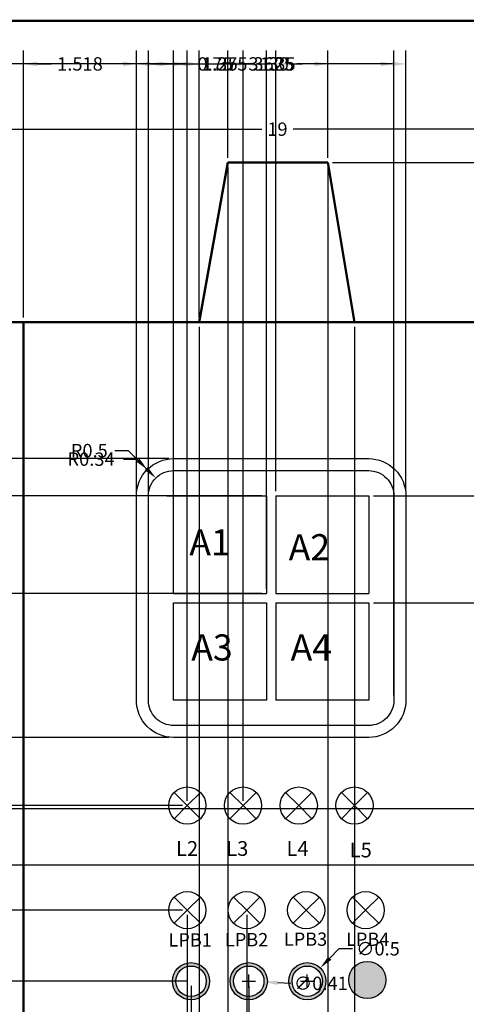
# Model space of a CAD drawing. Units: inches. Extents: x 0 to 33.5, y 0 to 22.4.
# Tile 3 of 6: x 10.7 to 16.8, y 9.2 to 22.4. Entities that reach past the tile are written whole.
import ezdxf
from ezdxf.enums import TextEntityAlignment as Align

# ---------------------------------------------------------------- set-up
doc = ezdxf.new("R2010")
doc.units = ezdxf.units.IN
doc.header["$MEASUREMENT"] = 0
for name, color, linetype, lineweight in [('E-ANNO-DIMS', 2, 'Continuous', 18), ('E-ANNO-TEXT', 7, 'Continuous', 18), ('E-ANNO-TTLB', 7, 'Continuous', 35), ('E-PANL-DEVC', 4, 'Continuous', 25), ('E-PANL-OUTL', 7, 'Continuous', 50), ('E-PANL-PATT', 8, 'Continuous', 13)]:
    doc.layers.add(name, color=color, linetype=linetype, lineweight=lineweight)
doc.layers.add('TITLE', color=7, linetype='Continuous')
doc.styles.add('ITALIC', font='ITALIC')
doc.styles.add('SIMPLEX', font='SIMPLEX')
doc.dimstyles.get("Standard").update_dxf_attribs({"dimtxt": 0.18, "dimasz": 0.18, "dimexe": 0.18, "dimexo": 0.0625, "dimgap": 0.09, "dimtad": 0, "dimtih": 1, "dimtoh": 1, "dimdec": 0, "dimzin": 0, "dimdsep": 46, "dimtxsty": 'Standard', "dimcen": 0.09, "dimadec": 0, "dimazin": 0, "dimtfac": 1, "dimtdec": 0, "dimtofl": 0, "dimtmove": 0, "dimatfit": 3, "dimfxl": 1, "dimtolj": 1, "dimtzin": 0, "dimarcsym": 0})

# ---------------------------------------------------------------- blocks, each defined once
blk = doc.blocks.new('NO_NUM_acade_title')
at = {"layer": 'TITLE', "const_width": 0.0312}
blk.add_lwpolyline([(30.594, 0.281), (30.594, 22.177), (30.344, 22.427), (0.281, 22.427), (0.031, 22.177), (0.031, 0.281), (0.281, 0.031), (30.344, 0.031)], close=True, dxfattribs=at)
at = {"layer": 'TITLE', "style": 'ITALIC'}
for tag, height, p in [('TITLE#1', 0.125, (32.156, 3.406)), ('TITLE#2', 0.125, (32.156, 3.204)), ('TITLE#3', 0.125, (32.156, 3.001)), ('TITLE#4', 0.125, (32.156, 2.799)), ('DWG#', 0.2, (32.156, 0.826))]:
    blk.add_attdef(tag, text='', height=height, dxfattribs=at).set_placement(p, align=Align.CENTER)
at = {"layer": 'TITLE', "style": 'SIMPLEX'}
blk.add_attdef('CAD#', (30.826, 1.958), '', height=0.0938, rotation=90, dxfattribs=at)
at = {"layer": 'TITLE'}
for tag, p, height, style in [('JOB#', (31.464, 1.644), 0.0938, 'SIMPLEX'), ('SCALE', (31.353, 1.344), 0.0938, 'SIMPLEX'), ('DATE', (32.408, 1.344), 0.0938, 'SIMPLEX'), ('SHTS', (32.532, 0.25), 0.2, 'ITALIC')]:
    blk.add_attdef(tag, p, '', height=height, dxfattribs=dict(at, style=style))
at = {"layer": 'TITLE', "style": 'ITALIC'}
blk.add_attdef('SH#', text='', height=0.2, dxfattribs=at).set_placement((31.881, 0.25), align=Align.RIGHT)
at = {"layer": 'TITLE', "flags": 9}
blk.add_attdef('WD_TB', (31.219, 0.031), '', height=0.125, dxfattribs=at)
blk = doc.blocks.new('*U7')
for q in [(-0.177, 0.177), (0.177, 0.177), (-0.177, -0.177), (0.177, -0.177)]:
    blk.add_line((0, 0), q)
blk.add_circle((0, 0), 0.25)
blk = doc.blocks.new('*U8')
at = {"layer": 'E-PANL-DEVC', "color": 0, "linetype": 'ByBlock', "lineweight": -2, "transparency": 16777216}
for p in [(0, 0), (0.75, 0), (1.5, 0), (2.25, 0)]:
    blk.add_blockref('*U7', p, dxfattribs=at)
blk = doc.blocks.new('*U11')
for q in [(-0.177, 0.177), (0.177, 0.177), (-0.177, -0.177), (0.177, -0.177)]:
    blk.add_line((0, 0), q)
blk.add_circle((0, 0), 0.25)
blk = doc.blocks.new('*U12')
at = {"layer": 'E-PANL-DEVC', "color": 0, "linetype": 'ByBlock', "lineweight": -2, "transparency": 16777216}
for p in [(0, 0), (0.8, 0), (1.6, 0), (2.4, 0)]:
    blk.add_blockref('*U11', p, dxfattribs=at)
blk = doc.blocks.new('*D18')
at = {"layer": 'Defpoints', "color": 0, "transparency": 16777216}
for p in [(23.794, 20.97), (4.625, 18.375), (23.794, 18.375)]:
    blk.add_point(p, dxfattribs=at)
at = {"layer": 'E-ANNO-DIMS', "color": 0, "lineweight": -2, "transparency": 16777216}
for p, q in [((4.625, 18.438), (4.625, 21.15)), ((23.794, 18.438), (23.794, 21.15)), ((4.805, 20.97), (13.999, 20.97)), ((23.614, 20.97), (14.419, 20.97))]:
    blk.add_line(p, q, dxfattribs=at)
at = {"layer": 'E-ANNO-DIMS', "color": 0, "transparency": 16777216}
for points in [[(4.805, 21), (4.805, 20.94), (4.625, 20.97)], [(23.614, 21), (23.614, 20.94), (23.794, 20.97)]]:
    blk.add_solid(points, dxfattribs=at)
at = {"layer": 'E-ANNO-DIMS', "color": 0, "transparency": 16777216, "insert": (14.209, 20.97), "char_height": 0.18, "attachment_point": 5}
blk.add_mtext('\\A1;19', dxfattribs=at)
blk = doc.blocks.new('PB-FLUSH')
for radius in [0.25, 0.205]:
    blk.add_circle((0.25, 0.25), radius)
blk = doc.blocks.new('*D26')
at = {"layer": 'Defpoints', "color": 0, "transparency": 16777216}
for p in [(14.887335, 21.847539), (13.540199, 20.522539), (14.887335, 20.522539)]:
    blk.add_point(p, dxfattribs=at)
at = {"layer": 'E-ANNO-DIMS', "color": 0, "lineweight": -2, "transparency": 16777216}
for p, q in [((13.540199, 20.585039), (13.540199, 22.027539)), ((14.887335, 20.585039), (14.887335, 22.027539)), ((13.720199, 21.847539), (13.883767, 21.847539)), ((14.707335, 21.847539), (14.543767, 21.847539))]:
    blk.add_line(p, q, dxfattribs=at)
at = {"layer": 'E-ANNO-DIMS', "color": 0, "transparency": 16777216}
for points in [[(13.720199, 21.877539), (13.720199, 21.817539), (13.540199, 21.847539)], [(14.707335, 21.877539), (14.707335, 21.817539), (14.887335, 21.847539)]]:
    blk.add_solid(points, dxfattribs=at)
at = {"layer": 'E-ANNO-DIMS', "color": 0, "transparency": 16777216, "insert": (14.213767, 21.847539), "char_height": 0.18, "attachment_point": 5}
blk.add_mtext('\\A1;1.35', dxfattribs=at)
blk = doc.blocks.new('*D27')
at = {"layer": 'Defpoints', "color": 0, "transparency": 16777216}
for p in [(13.540199, 20.522539), (13.156258, 18.375), (13.540199, 0.354641)]:
    blk.add_point(p, dxfattribs=at)
at = {"layer": 'E-ANNO-DIMS', "color": 0, "lineweight": -2, "transparency": 16777216}
for p, q in [((13.540199, 20.460039), (13.540199, 0.174641)), ((13.156258, 18.3125), (13.156258, 0.174641)), ((12.976258, 0.354641), (12.796258, 0.354641)), ((13.720199, 0.354641), (13.900199, 0.354641))]:
    blk.add_line(p, q, dxfattribs=at)
at = {"layer": 'E-ANNO-DIMS', "color": 0, "transparency": 16777216}
for points in [[(12.976258, 0.384641), (12.976258, 0.324641), (13.156258, 0.354641)], [(13.720199, 0.384641), (13.720199, 0.324641), (13.540199, 0.354641)]]:
    blk.add_solid(points, dxfattribs=at)
at = {"layer": 'E-ANNO-DIMS', "color": 0, "transparency": 16777216, "insert": (14.335199, 0.354641), "char_height": 0.18, "attachment_point": 5}
blk.add_mtext('\\A1;0.384', dxfattribs=at)
blk = doc.blocks.new('*D28')
at = {"layer": 'Defpoints', "color": 0, "transparency": 16777216}
for p in [(14.887335, 20.522539), (15.245612, 18.375), (15.245612, 0.354641)]:
    blk.add_point(p, dxfattribs=at)
at = {"layer": 'E-ANNO-DIMS', "color": 0, "lineweight": -2, "transparency": 16777216}
for p, q in [((14.887335, 20.460039), (14.887335, 0.174641)), ((15.245612, 18.3125), (15.245612, 0.174641)), ((14.707335, 0.354641), (14.527335, 0.354641)), ((15.425612, 0.354641), (15.605612, 0.354641))]:
    blk.add_line(p, q, dxfattribs=at)
at = {"layer": 'E-ANNO-DIMS', "color": 0, "transparency": 16777216}
for points in [[(14.707335, 0.384641), (14.707335, 0.324641), (14.887335, 0.354641)], [(15.425612, 0.384641), (15.425612, 0.324641), (15.245612, 0.354641)]]:
    blk.add_solid(points, dxfattribs=at)
at = {"layer": 'E-ANNO-DIMS', "color": 0, "transparency": 16777216, "insert": (15.950612, 0.354641), "char_height": 0.18, "attachment_point": 5}
blk.add_mtext('\\A1;0.36', dxfattribs=at)
blk = doc.blocks.new('*D29')
at = {"layer": 'Defpoints', "color": 0, "transparency": 16777216}
for p in [(14.887, 20.523), (27.492, 20.523), (15.246, 18.375)]:
    blk.add_point(p, dxfattribs=at)
at = {"layer": 'E-ANNO-DIMS', "color": 0, "lineweight": -2, "transparency": 16777216}
for p, q in [((14.95, 20.523), (27.672, 20.523)), ((27.492, 20.343), (27.492, 19.629)), ((27.492, 18.555), (27.492, 19.269)), ((15.308, 18.375), (27.672, 18.375))]:
    blk.add_line(p, q, dxfattribs=at)
at = {"layer": 'E-ANNO-DIMS', "color": 0, "transparency": 16777216}
for points in [[(27.462, 20.343), (27.522, 20.343), (27.492, 20.523)], [(27.462, 18.555), (27.522, 18.555), (27.492, 18.375)]]:
    blk.add_solid(points, dxfattribs=at)
at = {"layer": 'E-ANNO-DIMS', "color": 0, "transparency": 16777216, "insert": (27.492, 19.449), "char_height": 0.18, "attachment_point": 5}
blk.add_mtext('\\A1;2.15', dxfattribs=at)
blk = doc.blocks.new('*D30')
at = {"layer": 'Defpoints', "color": 0, "transparency": 16777216}
for p in [(13.156258, 21.847539), (4.625144, 18.375), (13.156258, 18.375)]:
    blk.add_point(p, dxfattribs=at)
at = {"layer": 'E-ANNO-DIMS', "color": 0, "lineweight": -2, "transparency": 16777216}
for p, q in [((4.625144, 18.4375), (4.625144, 22.027539)), ((13.156258, 18.4375), (13.156258, 22.027539)), ((4.805144, 21.847539), (8.470701, 21.847539)), ((12.976258, 21.847539), (9.310701, 21.847539))]:
    blk.add_line(p, q, dxfattribs=at)
at = {"layer": 'E-ANNO-DIMS', "color": 0, "transparency": 16777216}
for points in [[(4.805144, 21.877539), (4.805144, 21.817539), (4.625144, 21.847539)], [(12.976258, 21.877539), (12.976258, 21.817539), (13.156258, 21.847539)]]:
    blk.add_solid(points, dxfattribs=at)
at = {"layer": 'E-ANNO-DIMS', "color": 0, "transparency": 16777216, "insert": (8.890701, 21.847539), "char_height": 0.18, "attachment_point": 5}
blk.add_mtext('\\A1;8.531', dxfattribs=at)
blk = doc.blocks.new('*D31')
at = {"layer": 'Defpoints', "color": 0, "transparency": 16777216}
for p in [(14.887335, 20.522539), (27.49197, 20.522539), (23.941819, 1.679641)]:
    blk.add_point(p, dxfattribs=at)
at = {"layer": 'E-ANNO-DIMS', "color": 0, "lineweight": -2, "transparency": 16777216}
for p, q in [((14.949835, 20.522539), (27.67197, 20.522539)), ((27.49197, 20.342539), (27.49197, 11.28109)), ((27.49197, 1.859641), (27.49197, 10.92109)), ((24.004319, 1.679641), (27.67197, 1.679641))]:
    blk.add_line(p, q, dxfattribs=at)
at = {"layer": 'E-ANNO-DIMS', "color": 0, "transparency": 16777216}
for points in [[(27.46197, 20.342539), (27.52197, 20.342539), (27.49197, 20.522539)], [(27.46197, 1.859641), (27.52197, 1.859641), (27.49197, 1.679641)]]:
    blk.add_solid(points, dxfattribs=at)
at = {"layer": 'E-ANNO-DIMS', "color": 0, "transparency": 16777216, "insert": (27.49197, 11.10109), "char_height": 0.18, "attachment_point": 5}
blk.add_mtext('\\A1;18.843', dxfattribs=at)
blk = doc.blocks.new('*D51')
at = {"layer": 'Defpoints', "color": 0, "transparency": 16777216}
for p in [(15.936773, 21.847539), (12.311773, 16.038508), (15.936773, 16.038508)]:
    blk.add_point(p, dxfattribs=at)
at = {"layer": 'E-ANNO-DIMS', "color": 0, "lineweight": -2, "transparency": 16777216}
for p, q in [((12.311773, 16.101008), (12.311773, 22.027539)), ((15.936773, 16.101008), (15.936773, 22.027539)), ((12.491773, 21.847539), (13.674273, 21.847539)), ((15.756773, 21.847539), (14.574273, 21.847539))]:
    blk.add_line(p, q, dxfattribs=at)
at = {"layer": 'E-ANNO-DIMS', "color": 0, "transparency": 16777216}
for points in [[(12.491773, 21.877539), (12.491773, 21.817539), (12.311773, 21.847539)], [(15.756773, 21.877539), (15.756773, 21.817539), (15.936773, 21.847539)]]:
    blk.add_solid(points, dxfattribs=at)
at = {"layer": 'E-ANNO-DIMS', "color": 0, "transparency": 16777216, "insert": (14.124273, 21.847539), "char_height": 0.18, "attachment_point": 5}
blk.add_mtext('\\A1;3.625', dxfattribs=at)
blk = doc.blocks.new('*D52')
at = {"layer": 'Defpoints', "color": 0, "transparency": 16777216}
for p in [(15.775588, 21.847539), (12.472958, 13.288508), (15.775588, 13.288508)]:
    blk.add_point(p, dxfattribs=at)
at = {"layer": 'E-ANNO-DIMS', "color": 0, "lineweight": -2, "transparency": 16777216}
for p, q in [((12.472958, 13.351008), (12.472958, 22.027539)), ((15.775588, 13.351008), (15.775588, 22.027539)), ((12.652958, 21.847539), (13.779273, 21.847539)), ((15.595588, 21.847539), (14.469273, 21.847539))]:
    blk.add_line(p, q, dxfattribs=at)
at = {"layer": 'E-ANNO-DIMS', "color": 0, "transparency": 16777216}
for points in [[(12.652958, 21.877539), (12.652958, 21.817539), (12.472958, 21.847539)], [(15.595588, 21.877539), (15.595588, 21.817539), (15.775588, 21.847539)]]:
    blk.add_solid(points, dxfattribs=at)
at = {"layer": 'E-ANNO-DIMS', "color": 0, "transparency": 16777216, "insert": (14.124273, 21.847539), "char_height": 0.18, "attachment_point": 5}
blk.add_mtext('\\A1;3.30', dxfattribs=at)
blk = doc.blocks.new('*D53')
at = {"layer": 'Defpoints', "color": 0, "transparency": 16777216}
for p in [(14.061773, 21.847539), (12.811773, 14.726008), (14.061773, 14.726008)]:
    blk.add_point(p, dxfattribs=at)
at = {"layer": 'E-ANNO-DIMS', "color": 0, "lineweight": -2, "transparency": 16777216}
for p, q in [((12.811773, 14.788508), (12.811773, 22.027539)), ((14.061773, 14.788508), (14.061773, 22.027539)), ((12.991773, 21.847539), (13.106773, 21.847539)), ((13.881773, 21.847539), (13.766773, 21.847539))]:
    blk.add_line(p, q, dxfattribs=at)
at = {"layer": 'E-ANNO-DIMS', "color": 0, "transparency": 16777216}
for points in [[(12.991773, 21.877539), (12.991773, 21.817539), (12.811773, 21.847539)], [(13.881773, 21.877539), (13.881773, 21.817539), (14.061773, 21.847539)]]:
    blk.add_solid(points, dxfattribs=at)
at = {"layer": 'E-ANNO-DIMS', "color": 0, "transparency": 16777216, "insert": (13.436773, 21.847539), "char_height": 0.18, "attachment_point": 5}
blk.add_mtext('\\A1;1.25', dxfattribs=at)
blk = doc.blocks.new('*D54')
at = {"layer": 'Defpoints', "color": 0, "transparency": 16777216}
for p in [(14.061773, 16.038508), (1.272879, 14.726008), (14.061773, 14.726008)]:
    blk.add_point(p, dxfattribs=at)
at = {"layer": 'E-ANNO-DIMS', "color": 0, "lineweight": -2, "transparency": 16777216}
for p, q in [((13.999273, 16.038508), (1.092879, 16.038508)), ((1.272879, 15.858508), (1.272879, 15.562258)), ((1.272879, 14.906008), (1.272879, 15.202258)), ((13.999273, 14.726008), (1.092879, 14.726008))]:
    blk.add_line(p, q, dxfattribs=at)
at = {"layer": 'E-ANNO-DIMS', "color": 0, "transparency": 16777216}
for points in [[(1.242879, 15.858508), (1.302879, 15.858508), (1.272879, 16.038508)], [(1.242879, 14.906008), (1.302879, 14.906008), (1.272879, 14.726008)]]:
    blk.add_solid(points, dxfattribs=at)
at = {"layer": 'E-ANNO-DIMS', "color": 0, "transparency": 16777216, "insert": (1.272879, 15.382258), "char_height": 0.18, "attachment_point": 5}
blk.add_mtext('\\A1;1.31', dxfattribs=at)
blk = doc.blocks.new('*D55')
at = {"layer": 'Defpoints', "color": 0, "transparency": 16777216}
for p in [(14.186773, 21.847539), (12.811773, 16.038508), (14.186773, 16.038508)]:
    blk.add_point(p, dxfattribs=at)
at = {"layer": 'E-ANNO-DIMS', "color": 0, "lineweight": -2, "transparency": 16777216}
for p, q in [((12.811773, 16.101008), (12.811773, 22.027539)), ((14.186773, 16.101008), (14.186773, 22.027539)), ((12.631773, 21.847539), (12.451773, 21.847539)), ((14.366773, 21.847539), (14.546773, 21.847539))]:
    blk.add_line(p, q, dxfattribs=at)
at = {"layer": 'E-ANNO-DIMS', "color": 0, "transparency": 16777216}
for points in [[(12.631773, 21.877539), (12.631773, 21.817539), (12.811773, 21.847539)], [(14.366773, 21.877539), (14.366773, 21.817539), (14.186773, 21.847539)]]:
    blk.add_solid(points, dxfattribs=at)
at = {"layer": 'E-ANNO-DIMS', "color": 0, "transparency": 16777216, "insert": (13.499273, 21.847539), "char_height": 0.18, "attachment_point": 5}
blk.add_mtext('\\A1;1.375', dxfattribs=at)
blk = doc.blocks.new('*D56')
at = {"layer": 'Defpoints', "color": 0, "transparency": 16777216}
for p in [(15.436773, 16.038508), (15.436773, 14.601008), (27.49197, 14.601008)]:
    blk.add_point(p, dxfattribs=at)
at = {"layer": 'E-ANNO-DIMS', "color": 0, "lineweight": -2, "transparency": 16777216}
for p, q in [((15.499273, 16.038508), (27.67197, 16.038508)), ((27.49197, 15.858508), (27.49197, 15.499758)), ((27.49197, 14.781008), (27.49197, 15.139758)), ((15.499273, 14.601008), (27.67197, 14.601008))]:
    blk.add_line(p, q, dxfattribs=at)
at = {"layer": 'E-ANNO-DIMS', "color": 0, "transparency": 16777216}
for points in [[(27.46197, 15.858508), (27.52197, 15.858508), (27.49197, 16.038508)], [(27.46197, 14.781008), (27.52197, 14.781008), (27.49197, 14.601008)]]:
    blk.add_solid(points, dxfattribs=at)
at = {"layer": 'E-ANNO-DIMS', "color": 0, "transparency": 16777216, "insert": (27.49197, 15.319758), "char_height": 0.18, "attachment_point": 5}
blk.add_mtext('\\A1;1.44', dxfattribs=at)
blk = doc.blocks.new('*D57')
at = {"layer": 'Defpoints', "color": 0, "transparency": 16777216}
for p in [(12.312, 21.848), (10.794, 18.375), (12.312, 16.039)]:
    blk.add_point(p, dxfattribs=at)
at = {"layer": 'E-ANNO-DIMS', "color": 0, "lineweight": -2, "transparency": 16777216}
for p, q in [((10.794, 18.438), (10.794, 22.028)), ((12.312, 16.101), (12.312, 22.028)), ((10.974, 21.848), (11.163, 21.848)), ((12.132, 21.848), (11.943, 21.848))]:
    blk.add_line(p, q, dxfattribs=at)
at = {"layer": 'E-ANNO-DIMS', "color": 0, "transparency": 16777216}
for points in [[(10.974, 21.878), (10.974, 21.818), (10.794, 21.848)], [(12.132, 21.878), (12.132, 21.818), (12.312, 21.848)]]:
    blk.add_solid(points, dxfattribs=at)
at = {"layer": 'E-ANNO-DIMS', "color": 0, "transparency": 16777216, "insert": (11.553, 21.848), "char_height": 0.18, "attachment_point": 5}
blk.add_mtext('\\A1;1.518', dxfattribs=at)
blk = doc.blocks.new('*D58')
at = {"layer": 'Defpoints', "color": 0, "transparency": 16777216}
for p in [(10.794, 18.375), (12.996, 10.465), (12.996, 0.355)]:
    blk.add_point(p, dxfattribs=at)
at = {"layer": 'E-ANNO-DIMS', "color": 0, "lineweight": -2, "transparency": 16777216}
for p, q in [((10.794, 18.312), (10.794, 0.175)), ((12.996, 10.403), (12.996, 0.175)), ((10.974, 0.355), (11.46, 0.355)), ((12.816, 0.355), (12.33, 0.355))]:
    blk.add_line(p, q, dxfattribs=at)
at = {"layer": 'E-ANNO-DIMS', "color": 0, "transparency": 16777216}
for points in [[(10.974, 0.385), (10.974, 0.325), (10.794, 0.355)], [(12.816, 0.385), (12.816, 0.325), (12.996, 0.355)]]:
    blk.add_solid(points, dxfattribs=at)
at = {"layer": 'E-ANNO-DIMS', "color": 0, "transparency": 16777216, "insert": (11.895, 0.355), "char_height": 0.18, "attachment_point": 5}
blk.add_mtext('\\A1;2.202', dxfattribs=at)
blk = doc.blocks.new('*D59')
at = {"layer": 'Defpoints', "color": 0, "transparency": 16777216}
for p in [(10.793806, 18.375), (1.272879, 16.538508), (12.811773, 16.538508)]:
    blk.add_point(p, dxfattribs=at)
at = {"layer": 'E-ANNO-DIMS', "color": 0, "lineweight": -2, "transparency": 16777216}
for p, q in [((10.731306, 18.375), (1.092879, 18.375)), ((1.272879, 18.195), (1.272879, 17.636754)), ((1.272879, 16.718508), (1.272879, 17.276754)), ((12.749273, 16.538508), (1.092879, 16.538508))]:
    blk.add_line(p, q, dxfattribs=at)
at = {"layer": 'E-ANNO-DIMS', "color": 0, "transparency": 16777216}
for points in [[(1.242879, 18.195), (1.302879, 18.195), (1.272879, 18.375)], [(1.242879, 16.718508), (1.302879, 16.718508), (1.272879, 16.538508)]]:
    blk.add_solid(points, dxfattribs=at)
at = {"layer": 'E-ANNO-DIMS', "color": 0, "transparency": 16777216, "insert": (1.272879, 17.456754), "char_height": 0.18, "attachment_point": 5}
blk.add_mtext('\\A1;1.84', dxfattribs=at)
blk = doc.blocks.new('*D60')
at = {"layer": 'Defpoints', "color": 0, "transparency": 16777216}
for p in [(12.811773, 16.538508), (1.272879, 12.788508), (12.811773, 12.788508)]:
    blk.add_point(p, dxfattribs=at)
at = {"layer": 'E-ANNO-DIMS', "color": 0, "lineweight": -2, "transparency": 16777216}
for p, q in [((12.749273, 16.538508), (1.092879, 16.538508)), ((1.272879, 16.358508), (1.272879, 14.843508)), ((1.272879, 12.968508), (1.272879, 14.483508)), ((12.749273, 12.788508), (1.092879, 12.788508))]:
    blk.add_line(p, q, dxfattribs=at)
at = {"layer": 'E-ANNO-DIMS', "color": 0, "transparency": 16777216}
for points in [[(1.242879, 16.358508), (1.302879, 16.358508), (1.272879, 16.538508)], [(1.242879, 12.968508), (1.302879, 12.968508), (1.272879, 12.788508)]]:
    blk.add_solid(points, dxfattribs=at)
at = {"layer": 'E-ANNO-DIMS', "color": 0, "transparency": 16777216, "insert": (1.272879, 14.663508), "char_height": 0.18, "attachment_point": 5}
blk.add_mtext('\\A1;3.75', dxfattribs=at)
blk = doc.blocks.new('*D61')
at = {"layer": 'Defpoints', "color": 0, "transparency": 16777216}
for p in [(12.812, 12.789), (1.273, 11.873), (12.996, 11.873)]:
    blk.add_point(p, dxfattribs=at)
at = {"layer": 'E-ANNO-DIMS', "color": 0, "lineweight": -2, "transparency": 16777216}
for p, q in [((12.749, 12.789), (1.093, 12.789)), ((1.273, 12.609), (1.273, 12.511)), ((1.273, 12.053), (1.273, 12.151)), ((12.933, 11.873), (1.093, 11.873))]:
    blk.add_line(p, q, dxfattribs=at)
at = {"layer": 'E-ANNO-DIMS', "color": 0, "transparency": 16777216}
for points in [[(1.243, 12.609), (1.303, 12.609), (1.273, 12.789)], [(1.243, 12.053), (1.303, 12.053), (1.273, 11.873)]]:
    blk.add_solid(points, dxfattribs=at)
at = {"layer": 'E-ANNO-DIMS', "color": 0, "transparency": 16777216, "insert": (1.273, 12.331), "char_height": 0.18, "attachment_point": 5}
blk.add_mtext('\\A1;0.92', dxfattribs=at)
blk = doc.blocks.new('*D62')
at = {"layer": 'Defpoints', "color": 0, "transparency": 16777216}
for p in [(12.996, 11.873), (1.273, 10.465), (12.996, 10.465)]:
    blk.add_point(p, dxfattribs=at)
at = {"layer": 'E-ANNO-DIMS', "color": 0, "lineweight": -2, "transparency": 16777216}
for p, q in [((12.933, 11.873), (1.093, 11.873)), ((1.273, 11.693), (1.273, 11.349)), ((1.273, 10.645), (1.273, 10.989)), ((12.933, 10.465), (1.093, 10.465))]:
    blk.add_line(p, q, dxfattribs=at)
at = {"layer": 'E-ANNO-DIMS', "color": 0, "transparency": 16777216}
for points in [[(1.243, 11.693), (1.303, 11.693), (1.273, 11.873)], [(1.243, 10.645), (1.303, 10.645), (1.273, 10.465)]]:
    blk.add_solid(points, dxfattribs=at)
at = {"layer": 'E-ANNO-DIMS', "color": 0, "transparency": 16777216, "insert": (1.273, 11.169), "char_height": 0.18, "attachment_point": 5}
blk.add_mtext('\\A1;1.41', dxfattribs=at)
blk = doc.blocks.new('*D63')
at = {"layer": 'Defpoints', "color": 0, "transparency": 16777216}
for p in [(12.995825, 10.465374), (1.272879, 9.509708), (13.047227, 9.509708)]:
    blk.add_point(p, dxfattribs=at)
at = {"layer": 'E-ANNO-DIMS', "color": 0, "lineweight": -2, "transparency": 16777216}
for p, q in [((12.933325, 10.465374), (1.092879, 10.465374)), ((1.272879, 10.285374), (1.272879, 10.167541)), ((1.272879, 9.689708), (1.272879, 9.807541)), ((12.984727, 9.509708), (1.092879, 9.509708))]:
    blk.add_line(p, q, dxfattribs=at)
at = {"layer": 'E-ANNO-DIMS', "color": 0, "transparency": 16777216}
for points in [[(1.242879, 10.285374), (1.302879, 10.285374), (1.272879, 10.465374)], [(1.242879, 9.689708), (1.302879, 9.689708), (1.272879, 9.509708)]]:
    blk.add_solid(points, dxfattribs=at)
at = {"layer": 'E-ANNO-DIMS', "color": 0, "transparency": 16777216, "insert": (1.272879, 9.987541), "char_height": 0.18, "attachment_point": 5}
blk.add_mtext('\\A1;0.96', dxfattribs=at)
blk = doc.blocks.new('*D64')
at = {"layer": 'Defpoints', "color": 0, "transparency": 16777216}
for p in [(13.745825, 21.847539), (12.995825, 11.872685), (13.745825, 11.872685)]:
    blk.add_point(p, dxfattribs=at)
at = {"layer": 'E-ANNO-DIMS', "color": 0, "lineweight": -2, "transparency": 16777216}
for p, q in [((12.995825, 11.935185), (12.995825, 22.027539)), ((13.745825, 11.935185), (13.745825, 22.027539)), ((12.815825, 21.847539), (12.635825, 21.847539)), ((13.925825, 21.847539), (14.105825, 21.847539))]:
    blk.add_line(p, q, dxfattribs=at)
at = {"layer": 'E-ANNO-DIMS', "color": 0, "transparency": 16777216}
for points in [[(12.815825, 21.877539), (12.815825, 21.817539), (12.995825, 21.847539)], [(13.925825, 21.877539), (13.925825, 21.817539), (13.745825, 21.847539)]]:
    blk.add_solid(points, dxfattribs=at)
at = {"layer": 'E-ANNO-DIMS', "color": 0, "transparency": 16777216, "insert": (13.370825, 21.847539), "char_height": 0.18, "attachment_point": 5}
blk.add_mtext('\\A1;0.75', dxfattribs=at)
blk = doc.blocks.new('*D65')
at = {"layer": 'Defpoints', "color": 0, "transparency": 16777216}
for p in [(12.995825, 10.465374), (13.795825, 10.465374), (13.795825, 0.354641)]:
    blk.add_point(p, dxfattribs=at)
at = {"layer": 'E-ANNO-DIMS', "color": 0, "lineweight": -2, "transparency": 16777216}
for p, q in [((12.995825, 10.402874), (12.995825, 0.174641)), ((13.795825, 10.402874), (13.795825, 0.174641)), ((13.175825, 0.354641), (13.615825, 0.354641)), ((13.795825, 0.354641), (13.975825, 0.354641))]:
    blk.add_line(p, q, dxfattribs=at)
at = {"layer": 'E-ANNO-DIMS', "color": 0, "transparency": 16777216}
for points in [[(13.175825, 0.384641), (13.175825, 0.324641), (12.995825, 0.354641)], [(13.615825, 0.384641), (13.615825, 0.324641), (13.795825, 0.354641)]]:
    blk.add_solid(points, dxfattribs=at)
at = {"layer": 'E-ANNO-DIMS', "color": 0, "transparency": 16777216, "insert": (14.230825, 0.354641), "char_height": 0.18, "attachment_point": 5}
blk.add_mtext('\\A1;0.8', dxfattribs=at)
blk = doc.blocks.new('*D66')
at = {"layer": 'Defpoints', "color": 0, "transparency": 16777216}
for p in [(13.047, 9.51), (13.823, 9.51), (13.823, 0.355)]:
    blk.add_point(p, dxfattribs=at)
at = {"layer": 'E-ANNO-DIMS', "color": 0, "lineweight": -2, "transparency": 16777216}
for p, q in [((13.047, 9.447), (13.047, 0.175)), ((13.823, 9.447), (13.823, 0.175)), ((12.867, 0.355), (12.687, 0.355)), ((14.003, 0.355), (14.183, 0.355))]:
    blk.add_line(p, q, dxfattribs=at)
at = {"layer": 'E-ANNO-DIMS', "color": 0, "transparency": 16777216}
for points in [[(12.867, 0.385), (12.867, 0.325), (13.047, 0.355)], [(14.003, 0.385), (14.003, 0.325), (13.823, 0.355)]]:
    blk.add_solid(points, dxfattribs=at)
at = {"layer": 'E-ANNO-DIMS', "color": 0, "transparency": 16777216, "insert": (13.435, 0.355), "char_height": 0.18, "attachment_point": 5}
blk.add_mtext('\\A1;0.78', dxfattribs=at)
blk = doc.blocks.new('*D86')
at = {"layer": 'Defpoints', "color": 0, "transparency": 16777216}
for p in [(19.972101, 11.828212), (1.272879, 11.072826), (19.972101, 11.072826)]:
    blk.add_point(p, dxfattribs=at)
at = {"layer": 'E-ANNO-DIMS', "color": 0, "lineweight": -2, "transparency": 16777216}
for p, q in [((19.909601, 11.828212), (1.092879, 11.828212)), ((1.272879, 11.648212), (1.272879, 11.252826)), ((19.909601, 11.072826), (1.092879, 11.072826)), ((1.272879, 11.072826), (1.272879, 10.892826)), ((1.272879, 10.892826), (1.092879, 10.892826))]:
    blk.add_line(p, q, dxfattribs=at)
at = {"layer": 'E-ANNO-DIMS', "color": 0, "transparency": 16777216}
for points in [[(1.242879, 11.648212), (1.302879, 11.648212), (1.272879, 11.828212)], [(1.242879, 11.252826), (1.302879, 11.252826), (1.272879, 11.072826)]]:
    blk.add_solid(points, dxfattribs=at)
at = {"layer": 'E-ANNO-DIMS', "color": 0, "transparency": 16777216, "insert": (0.747879, 10.892826), "char_height": 0.18, "attachment_point": 5}
blk.add_mtext('\\A1;0.76', dxfattribs=at)
blk = doc.blocks.new('*D91')
at = {"layer": 'Defpoints', "color": 0, "transparency": 16777216}
for p in [(12.458, 16.392), (12.812, 16.039)]:
    blk.add_point(p, dxfattribs=at)
at = {"layer": 'E-ANNO-DIMS', "color": 0, "lineweight": -2, "transparency": 16777216}
for p, q in [((12.023, 16.646), (12.203, 16.646)), ((12.203, 16.646), (12.331, 16.519)), ((12.722, 16.039), (12.902, 16.039)), ((12.812, 15.949), (12.812, 16.129))]:
    blk.add_line(p, q, dxfattribs=at)
at = {"layer": 'E-ANNO-DIMS', "color": 0, "transparency": 16777216}
blk.add_solid([(12.352, 16.54), (12.31, 16.498), (12.458, 16.392)], dxfattribs=at)
at = {"layer": 'E-ANNO-DIMS', "color": 0, "transparency": 16777216, "insert": (11.678, 16.646), "char_height": 0.18, "attachment_point": 5}
blk.add_mtext('\\A1;R0.5', dxfattribs=at)
blk = doc.blocks.new('*D92')
at = {"layer": 'Defpoints', "color": 0, "transparency": 16777216}
for p in [(12.572, 16.278), (12.812, 16.039)]:
    blk.add_point(p, dxfattribs=at)
at = {"layer": 'E-ANNO-DIMS', "color": 0, "lineweight": -2, "transparency": 16777216}
for p, q in [((12.137, 16.532), (12.317, 16.532)), ((12.317, 16.532), (12.445, 16.405)), ((12.722, 16.039), (12.902, 16.039)), ((12.812, 15.949), (12.812, 16.129))]:
    blk.add_line(p, q, dxfattribs=at)
at = {"layer": 'E-ANNO-DIMS', "color": 0, "transparency": 16777216}
blk.add_solid([(12.466, 16.426), (12.423, 16.384), (12.572, 16.278)], dxfattribs=at)
at = {"layer": 'E-ANNO-DIMS', "color": 0, "transparency": 16777216, "insert": (11.702, 16.532), "char_height": 0.18, "attachment_point": 5}
blk.add_mtext('\\A1;R0.34', dxfattribs=at)
blk = doc.blocks.new('*D93')
at = {"layer": 'Defpoints', "color": 0, "transparency": 16777216}
for p in [(13.619, 9.52), (14.028, 9.499)]:
    blk.add_point(p, dxfattribs=at)
at = {"layer": 'E-ANNO-DIMS', "color": 0, "lineweight": -2, "transparency": 16777216}
for p, q in [((13.823, 9.42), (13.823, 9.6)), ((13.733, 9.51), (13.913, 9.51)), ((14.388, 9.481), (14.208, 9.49))]:
    blk.add_line(p, q, dxfattribs=at)
at = {"layer": 'E-ANNO-DIMS', "color": 0, "transparency": 16777216}
blk.add_solid([(14.21, 9.52), (14.207, 9.46), (14.028, 9.499)], dxfattribs=at)
at = {"layer": 'E-ANNO-DIMS', "color": 0, "transparency": 16777216, "insert": (14.793, 9.481), "char_height": 0.18, "attachment_point": 5}
blk.add_mtext('\\A1;∅0.41', dxfattribs=at)
blk = doc.blocks.new('*D94')
at = {"layer": 'Defpoints', "color": 0, "transparency": 16777216}
for p in [(14.785, 9.689), (14.436, 9.331)]:
    blk.add_point(p, dxfattribs=at)
at = {"layer": 'E-ANNO-DIMS', "color": 0, "lineweight": -2, "transparency": 16777216}
for p, q in [((15.037, 9.946), (14.911, 9.817)), ((15.217, 9.946), (15.037, 9.946)), ((14.611, 9.42), (14.611, 9.6)), ((14.521, 9.51), (14.701, 9.51))]:
    blk.add_line(p, q, dxfattribs=at)
at = {"layer": 'E-ANNO-DIMS', "color": 0, "transparency": 16777216}
blk.add_solid([(14.89, 9.838), (14.933, 9.797), (14.785, 9.689)], dxfattribs=at)
at = {"layer": 'E-ANNO-DIMS', "color": 0, "transparency": 16777216, "insert": (15.562, 9.946), "char_height": 0.18, "attachment_point": 5}
blk.add_mtext('\\A1;∅0.5', dxfattribs=at)

msp = doc.modelspace()

# ---------------------------------------------------------------- hatches: boundary and pattern name
at = {"layer": 'E-PANL-PATT'}
h = msp.add_hatch(color=256, dxfattribs=at)
h.dxf.hatch_style = 1
h.paths.add_polyline_path([(9.0712, 10.6304, 1), (9.5712, 10.6304, 1)])
h.paths.add_polyline_path([(8.5702, 10.6304, 1), (8.0702, 10.6304, 1)])
h.paths.add_polyline_path([(8.115, 10.6304, -1), (8.5254, 10.6304, -1)], flags=16)
h.paths.add_polyline_path([(13.2972, 9.5097, 1), (12.7972, 9.5097, 1)])
h.paths.add_polyline_path([(12.842, 9.5097, -1), (13.2524, 9.5097, -1)], flags=16)
h = msp.add_hatch(color=256, dxfattribs=at)
h.dxf.hatch_style = 1
h.paths.add_polyline_path([(15.1694, 9.5269, 1), (15.6694, 9.5269, 1)])
h.paths.add_polyline_path([(14.8608, 9.5097, 1), (14.3608, 9.5097, 1)])
h.paths.add_polyline_path([(14.4056, 9.5097, -1), (14.816, 9.5097, -1)], flags=16)
h.paths.add_polyline_path([(14.0735, 9.5097, 1), (13.5735, 9.5097, 1)])
h.paths.add_polyline_path([(13.6183, 9.5097, -1), (14.0287, 9.5097, -1)], flags=16)

# ---------------------------------------------------------------- linework, layer by layer
at = {"layer": 'E-PANL-DEVC'}
for p, q in [((14.0618, 16.0385), (14.0618, 14.726)), ((14.1868, 16.0385), (14.1868, 14.726)), ((12.8118, 14.726), (14.0618, 14.726)), ((14.1868, 14.726), (15.4368, 14.726)), ((12.8118, 14.601), (14.0618, 14.601)), ((14.0618, 14.601), (14.0618, 13.2885)), ((14.1868, 14.601), (14.1868, 13.2885)), ((14.1868, 14.601), (15.4368, 14.601))]:
    msp.add_line(p, q, dxfattribs=at)
for points in [[(12.3118, 16.0385, -0.4142136), (12.8118, 16.5385), (15.4368, 16.5385, -0.4142136), (15.9368, 16.0385), (15.9368, 13.2885, -0.4142136), (15.4368, 12.7885), (12.8118, 12.7885, -0.4142136), (12.3118, 13.2885)], [(12.473, 16.0385, -0.4142136), (12.8118, 16.3773), (15.4368, 16.3773, -0.4142136), (15.7756, 16.0385), (15.7756, 13.2885, -0.4142136), (15.4368, 12.9497), (12.8118, 12.9497, -0.4142136), (12.473, 13.2885)]]:
    msp.add_lwpolyline(points, format="xyb", close=True, dxfattribs=at)
for points in [[(12.8118, 14.726), (12.8118, 16.0385), (14.0618, 16.0385)], [(14.1868, 16.0385), (15.4368, 16.0385), (15.4368, 14.726)], [(14.0618, 13.2885), (12.8118, 13.2885), (12.8118, 14.601)], [(15.4368, 14.601), (15.4368, 13.2885), (14.1868, 13.2885)]]:
    msp.add_lwpolyline(points, dxfattribs=at)
msp.add_circle((15.4194, 9.5269), 0.25, dxfattribs=at)
at = {"layer": 'E-PANL-OUTL'}
for p, q in [((13.5402, 20.5225), (13.1563, 18.375)), ((14.8873, 20.5225), (13.5402, 20.5225)), ((14.2094, 20.5225), (14.8873, 20.5225)), ((14.8873, 20.5225), (15.2456, 18.375)), ((4.6251, 18.375), (23.7937, 18.375)), ((10.7938, 3.5899), (10.7938, 18.375))]:
    msp.add_line(p, q, dxfattribs=at)

# ---------------------------------------------------------------- block references
at = {"layer": 'E-ANNO-TTLB'}
msp.add_blockref('NO_NUM_acade_title', (0, 0), dxfattribs=at)
at = {"layer": 'E-PANL-DEVC'}
for name, p in [('*U8', (12.9958, 11.8727)), ('*U12', (12.9958, 10.4654)), ('PB-FLUSH', (12.797, 9.2594)), ('PB-FLUSH', (13.5733, 9.2594)), ('PB-FLUSH', (14.3606, 9.2594))]:
    msp.add_blockref(name, p, dxfattribs=at)

# ---------------------------------------------------------------- texts
at = {"layer": 'E-ANNO-TEXT'}
for s, height, p in [('A1', 0.35114, (13.0238, 15.2364)), ('A2', 0.35114, (14.3602, 15.1716)), ('A3', 0.35114, (13.0498, 13.8235)), ('A4', 0.35114, (14.3862, 13.8235)), ('L2', 0.19791, (12.8457, 11.1962)), ('L3', 0.19791, (13.5209, 11.1962)), ('L4', 0.19791, (14.3308, 11.1962)), ('L5', 0.19791, (15.1821, 11.1754)), ('LPB1', 0.17877, (12.7436, 9.976)), ('LPB2', 0.17877, (13.5031, 9.9793)), ('LPB3', 0.17877, (14.2959, 9.986)), ('LPB4', 0.17877, (15.1323, 9.985))]:
    msp.add_text(s, height=height, dxfattribs=at).set_placement(p)

# ---------------------------------------------------------------- dimensions: what is measured, and where the dimension line sits
at = {"layer": 'E-ANNO-DIMS'}
for base, p1, p2, override, picture, middle in [((13.1563, 21.8475), (4.6251, 18.375), (13.1563, 18.375), {"dimdec": 3, "dimlfac": 1, "dimrnd": 0, "dimzin": 0, "dimdsep": 46, "dimlunit": 2}, '*D30', (8.8907, 21.8475)), ((12.3118, 21.8475), (10.7938, 18.375), (12.3118, 16.0385), {"dimdec": 3, "dimlfac": 1, "dimrnd": 0, "dimzin": 0, "dimdsep": 46, "dimlunit": 2}, '*D57', (11.5528, 21.8475)), ((15.9368, 21.8475), (12.3118, 16.0385), (15.9368, 16.0385), {"dimdec": 3, "dimlfac": 1, "dimrnd": 0, "dimzin": 0, "dimdsep": 46, "dimlunit": 2}, '*D51', (14.1243, 21.8475)), ((14.1868, 21.8475), (12.8118, 16.0385), (14.1868, 16.0385), {"dimdec": 3, "dimlfac": 1, "dimrnd": 0, "dimzin": 0, "dimdsep": 46, "dimlunit": 2}, '*D55', (13.4993, 21.8475)), ((15.7756, 21.8475), (12.473, 13.2885), (15.7756, 13.2885), {"dimdec": 2, "dimlfac": 1, "dimrnd": 0, "dimzin": 0, "dimdsep": 46, "dimlunit": 2}, '*D52', (14.1243, 21.8475)), ((13.7458, 21.8475), (12.9958, 11.8727), (13.7458, 11.8727), {"dimdec": 2, "dimlfac": 1, "dimrnd": 0, "dimzin": 0, "dimdsep": 46, "dimlunit": 2}, '*D64', (13.3708, 21.8475)), ((14.0618, 21.8475), (12.8118, 14.726), (14.0618, 14.726), {"dimdec": 2, "dimlfac": 1, "dimrnd": 0, "dimzin": 0, "dimdsep": 46, "dimlunit": 2}, '*D53', (13.4368, 21.8475)), ((14.8873, 21.8475), (13.5402, 20.5225), (14.8873, 20.5225), {"dimdec": 2, "dimlfac": 1, "dimrnd": 0, "dimzin": 0, "dimdsep": 46, "dimlunit": 2}, '*D26', (14.2138, 21.8475)), ((23.7937, 20.9702), (4.6251, 18.375), (23.7937, 18.375), {"dimclrd": 0, "dimclre": 0, "dimclrt": 0}, '*D18', (14.2094, 20.9702)), ((13.5402, 0.3546), (13.1563, 18.375), (13.5402, 20.5225), {"dimdec": 3, "dimlfac": 1, "dimrnd": 0, "dimzin": 0, "dimdsep": 46, "dimlunit": 2}, '*D27', (14.3352, 0.3546)), ((15.2456, 0.3546), (14.8873, 20.5225), (15.2456, 18.375), {"dimdec": 2, "dimlfac": 1, "dimrnd": 0, "dimzin": 0, "dimdsep": 46, "dimlunit": 2}, '*D28', (15.9506, 0.3546)), ((12.9958, 0.3546), (10.7938, 18.375), (12.9958, 10.4654), {"dimdec": 3, "dimlfac": 1, "dimrnd": 0, "dimzin": 0, "dimdsep": 46, "dimlunit": 2}, '*D58', (11.8948, 0.3546)), ((13.7958, 0.3546), (12.9958, 10.4654), (13.7958, 10.4654), {"dimdec": 1, "dimlfac": 1, "dimrnd": 0, "dimzin": 0, "dimdsep": 46, "dimlunit": 2}, '*D65', (14.2308, 0.3546)), ((13.8235, 0.3546), (13.0472, 9.5097), (13.8235, 9.5097), {"dimdec": 2, "dimlfac": 1, "dimrnd": 0, "dimzin": 0, "dimdsep": 46, "dimlunit": 2}, '*D66', (13.4354, 0.3546))]:
    dim = msp.add_linear_dim(base=base, p1=p1, p2=p2, dimstyle='Standard', override=override, dxfattribs=at)
    dim.commit()
    dim.dimension.update_dxf_attribs({"geometry": picture, "text_midpoint": middle})
for base, p1, p2, override, picture, middle in [((27.492, 20.5225), (15.2456, 18.375), (14.8873, 20.5225), {"dimdec": 2, "dimlfac": 1, "dimrnd": 0, "dimzin": 0, "dimdsep": 46, "dimlunit": 2}, '*D29', (27.492, 19.4488)), ((27.492, 20.5225), (23.9418, 1.6796), (14.8873, 20.5225), {"dimdec": 3, "dimlfac": 1, "dimrnd": 0, "dimzin": 0, "dimdsep": 46, "dimlunit": 2}, '*D31', (27.492, 11.1011)), ((1.2729, 16.5385), (10.7938, 18.375), (12.8118, 16.5385), {"dimdec": 2, "dimlfac": 1, "dimrnd": 0, "dimzin": 0, "dimdsep": 46, "dimlunit": 2}, '*D59', (1.2729, 17.4568)), ((1.2729, 12.7885), (12.8118, 16.5385), (12.8118, 12.7885), {"dimdec": 2, "dimlfac": 1, "dimrnd": 0, "dimzin": 0, "dimdsep": 46, "dimlunit": 2}, '*D60', (1.2729, 14.6635)), ((1.2729, 14.726), (14.0618, 16.0385), (14.0618, 14.726), {"dimdec": 2, "dimlfac": 1, "dimrnd": 0, "dimzin": 0, "dimdsep": 46, "dimlunit": 2}, '*D54', (1.2729, 15.3823)), ((27.492, 14.601), (15.4368, 16.0385), (15.4368, 14.601), {"dimdec": 2, "dimlfac": 1, "dimrnd": 0, "dimzin": 0, "dimdsep": 46, "dimlunit": 2}, '*D56', (27.492, 15.3198)), ((1.2729, 11.8727), (12.8118, 12.7885), (12.9958, 11.8727), {"dimdec": 2, "dimlfac": 1, "dimrnd": 0, "dimzin": 0, "dimdsep": 46, "dimlunit": 2}, '*D61', (1.2729, 12.3306)), ((1.2729, 11.0728), (19.9721, 11.8282), (19.9721, 11.0728), {"dimdec": 2, "dimlfac": 1, "dimrnd": 0, "dimzin": 0, "dimdsep": 46, "dimlunit": 2}, '*D86', (0.7479, 10.8928)), ((1.2729, 10.4654), (12.9958, 11.8727), (12.9958, 10.4654), {"dimdec": 2, "dimlfac": 1, "dimrnd": 0, "dimzin": 0, "dimdsep": 46, "dimlunit": 2}, '*D62', (1.2729, 11.169)), ((1.2729, 9.5097), (12.9958, 10.4654), (13.0472, 9.5097), {"dimdec": 2, "dimlfac": 1, "dimrnd": 0, "dimzin": 0, "dimdsep": 46, "dimlunit": 2}, '*D63', (1.2729, 9.9875))]:
    dim = msp.add_linear_dim(base=base, p1=p1, p2=p2, angle=90, dimstyle='Standard', override=override, dxfattribs=at)
    dim.commit()
    dim.dimension.update_dxf_attribs({"geometry": picture, "text_midpoint": middle})
for mpoint, override, picture, middle in [((12.4581, 16.3919), {"dimdec": 1, "dimlfac": 1, "dimrnd": 0, "dimzin": 0, "dimdsep": 46, "dimlunit": 2}, '*D91', (11.6784, 16.6464)), ((12.5721, 16.2779), {"dimdec": 2, "dimlfac": 1, "dimrnd": 0, "dimzin": 0, "dimdsep": 46, "dimlunit": 2}, '*D92', (11.7023, 16.5324))]:
    dim = msp.add_radius_dim(center=(12.8118, 16.0385), mpoint=mpoint, dimstyle='Standard', override=override, dxfattribs=at)
    dim.commit()
    dim.dimension.update_dxf_attribs({"geometry": picture, "text_midpoint": middle})
dim = msp.add_diameter_dim_2p(p1=(14.4362, 9.3308), p2=(14.7854, 9.6887), dimstyle='Standard', override={"dimdec": 1, "dimlfac": 1, "dimrnd": 0, "dimzin": 0, "dimdsep": 46, "dimlunit": 2}, dxfattribs=at)
dim.commit()
dim.dimension.update_dxf_attribs({"geometry": '*D94', "text_midpoint": (15.5618, 9.9463), "dimtype": 163})
dim = msp.add_diameter_dim_2p(p1=(13.6185, 9.5201), p2=(14.0284, 9.4993), dimstyle='Standard', override={"dimdec": 2, "dimlfac": 1, "dimrnd": 0, "dimzin": 0, "dimdsep": 46, "dimlunit": 2}, dxfattribs=at)
dim.commit()
dim.dimension.update_dxf_attribs({"geometry": '*D93', "text_midpoint": (14.388, 9.4811)})

doc.saveas('drawing.dxf')
